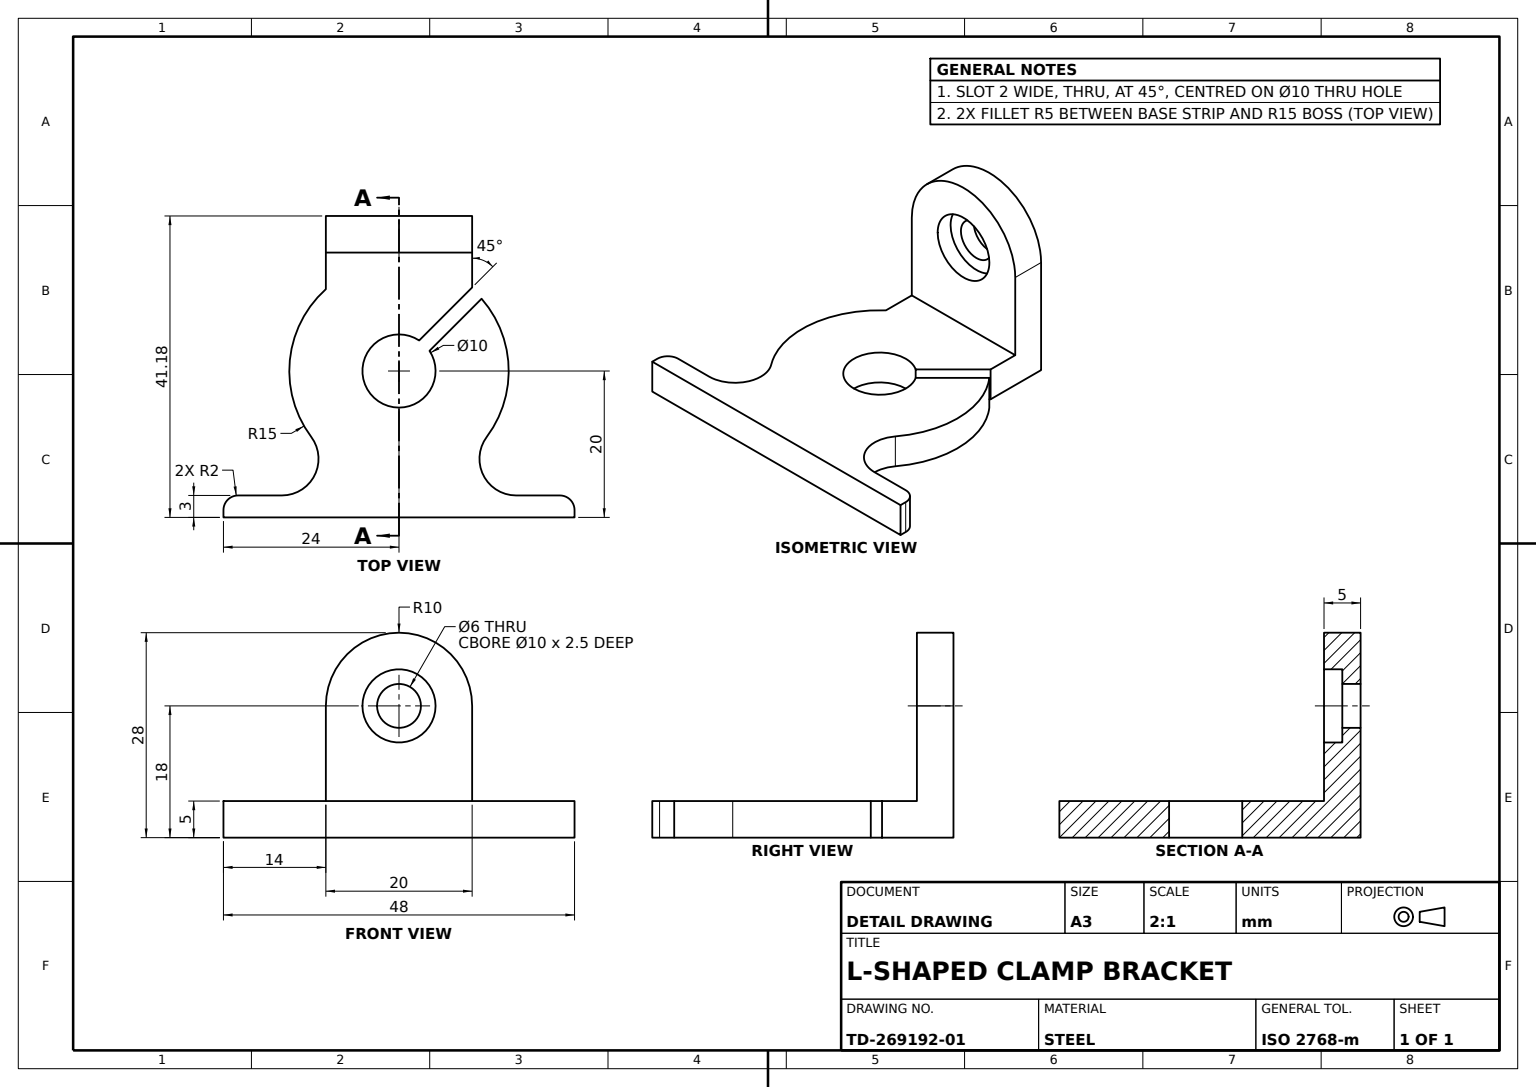
from build123d import *

# Parameters (mm, degrees)
BASE_PLATE_5MM_DEPTH           = 5
UPRIGHT_LUG_PROFILE_SKETCH_R   = 3
UPRIGHT_LUG_DEPTH              = 5
PIVOT_START                    = -2.5
PIVOT_COUNTERBORE_SKETCH_R     = 5
PIVOT_COUNTERBORE_SKETCH_R_2   = 3
PIVOT_COUNTERBORE_10X2_5_DEPTH = 2.5


with BuildPart() as part:
    # Base Plate Profile Sketch → Base Plate 5mm (new body)
    with BuildSketch(Plane(origin=(0, 0, 0), x_dir=(1, 0, 0), z_dir=(0, 1, 0))):
        with BuildLine():
            Line((-24, 1), (-24, 0))
            Line((-24, 0), (24, 0))
            Line((24, 0), (24, 1))
            ThreePointArc((24, 1), (23.414213562, 2.414213562), (22, 3))
            Line((22, 3), (16, 3))
            ThreePointArc((16, 3), (11.527864045, 5.763932023), (12, 11))
            ThreePointArc((12, 11), (14.989403432, 20.563724014), (11.290112025, 29.875898463))
            Line((11.290112025, 29.875898463), (4.171208396, 22.756994834))
            ThreePointArc((4.171208396, 22.756994834), (-3.535533906, 16.464466094), (2.756994834, 24.171208396))
            Line((2.756994834, 24.171208396), (10, 31.414213562))
            Line((10, 31.414213562), (10, 35))
            Line((10, 35), (10, 41.180339887))
            Line((10, 41.180339887), (-10, 41.180339887))
            Line((-10, 41.180339887), (-10, 35))
            Line((-10, 35), (-10, 31.180339887))
            ThreePointArc((-10, 31.180339887), (-14.92687273, 21.479348), (-12, 11))
            ThreePointArc((-12, 11), (-11.527864045, 5.763932023), (-16, 3))
            Line((-16, 3), (-22, 3))
            ThreePointArc((-22, 3), (-23.414213562, 2.414213562), (-24, 1))
        make_face()
    extrude(amount=BASE_PLATE_5MM_DEPTH)

    # Upright Lug Profile Sketch → Upright Lug (add)
    with BuildSketch(Plane(origin=(0, 0, -41.180339887), x_dir=(-1, 0, 0), z_dir=(0, 0, -1))):
        with BuildLine():
            Line((-10, 18), (-10, 0))
            Line((-10, 0), (10, 0))
            Line((10, 0), (10, 18))
            ThreePointArc((10, 18), (0, 28), (-10, 18))
        make_face()
        with Locations((0, 18)):
            Circle(UPRIGHT_LUG_PROFILE_SKETCH_R, mode=Mode.SUBTRACT)
    extrude(amount=-UPRIGHT_LUG_DEPTH)

    # Pivot Counterbore Sketch → Pivot Counterbore Ø10x2.5 (cut)
    with BuildSketch(Plane.XY.offset(-36.180339887).offset(PIVOT_START)):
        with Locations((0, 18)):
            Circle(PIVOT_COUNTERBORE_SKETCH_R)
        with Locations(Location((0, 18, 0), (0, 0, 180))):
            Circle(PIVOT_COUNTERBORE_SKETCH_R_2, mode=Mode.SUBTRACT)
    extrude(amount=PIVOT_COUNTERBORE_10X2_5_DEPTH, mode=Mode.SUBTRACT)


solid = part.part
